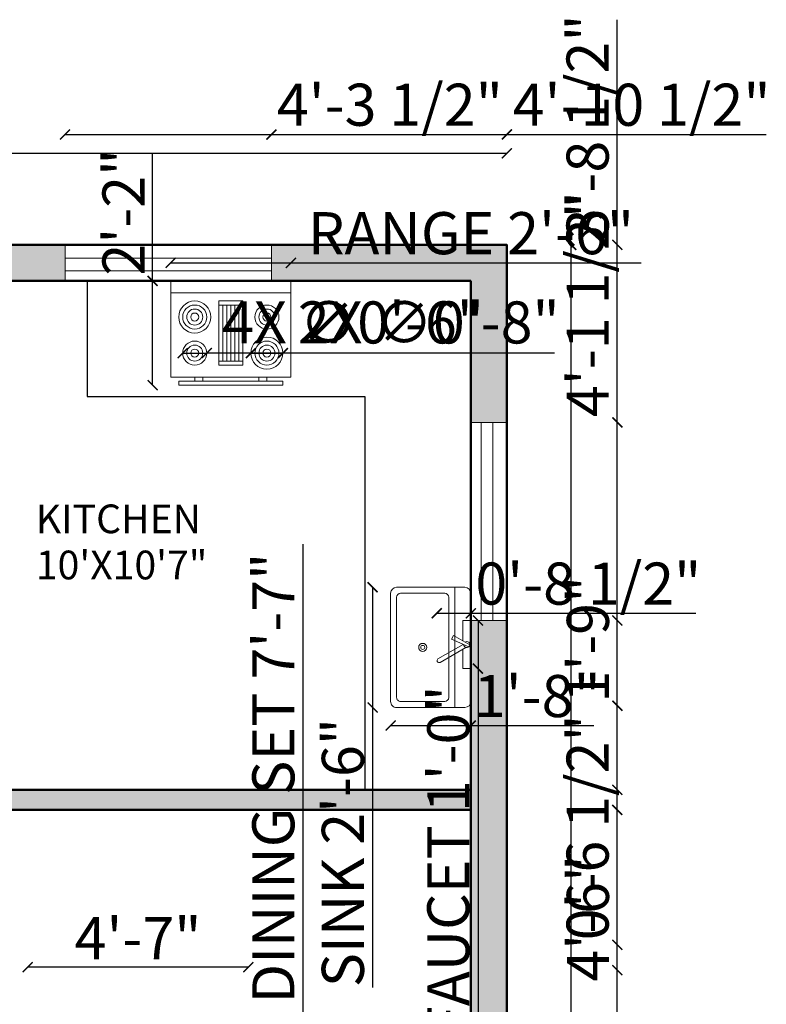
# Model space of a CAD drawing. Units: inches. Extents: x 1699 to 2290, y 1404 to 1978.
# Tile 4 of 4: x 2086 to 2273, y 1732 to 1978. Entities that reach past the tile are written whole.
import ezdxf

# ---------------------------------------------------------------- set-up
doc = ezdxf.new("R2010")
doc.units = ezdxf.units.IN
for name, color, linetype, lineweight in [('A-ANNO-DIMS', 2, 'Continuous', 18), ('A-AREA-IDEN', 7, 'Continuous', 25), ('A-EQPM', 8, 'Continuous', 18), ('A-FLOR-CASE', 8, 'Continuous', 25), ('A-FLOR-FIXT', 9, 'Continuous', 18), ('A-WALL', 7, 'Continuous', 50), ('A-WALL-PATT', 17, 'Continuous', 13), ('window', 3, 'Continuous', 18)]:
    doc.layers.add(name, color=color, linetype=linetype, lineweight=lineweight)
doc.styles.get("Standard").update_dxf_attribs({"font": 'arial.ttf'})
doc.dimstyles.new('ISO-25', dxfattribs={"dimtxt": 10.5, "dimasz": 2.5, "dimexe": 1.25, "dimexo": 0.625, "dimtad": 1, "dimdec": 0, "dimlunit": 4, "dimtxsty": 'Standard', "dimblk": 'ARCHTICK', "dimcen": 2.5, "dimse1": 1, "dimse2": 1, "dimclrd": 4, "dimclrt": 2, "dimadec": 0, "dimazin": 0, "dimtfac": 1, "dimtdec": 0, "dimtmove": 0, "dimatfit": 3, "dimfxl": 1, "dimarcsym": 0})

# ---------------------------------------------------------------- blocks, each defined once
blk = doc.blocks.new('Range-Oven - 30 in top')
for p, q in [((0, -3), (30, -3)), ((12, -6), (18, -6)), ((13, -20), (13, -6)), ((14, -6), (14, -20)), ((15, -20), (15, -6)), ((16, -6), (16, -20)), ((17, -20), (17, -6)), ((18, -20), (12, -20)), ((6, -24), (6, -25)), ((8, -25), (8, -24)), ((22, -25), (22, -24)), ((24, -24), (24, -25))]:
    blk.add_line(p, q)
for points in [[(0, -24), (0, 0), (30, 0), (30, -24)], [(12, -21), (12, -5), (18, -5), (18, -21)], [(2, -26), (2, -25), (28, -25), (28, -26)]]:
    blk.add_lwpolyline(points, close=True)
for centre, radius in [((6, -9), 4), ((6, -9), 3), ((6, -9), 2), ((24, -9), 3), ((24, -9), 2), ((6, -9), 1), ((24, -9), 1), ((24, -18), 4), ((6, -18), 3), ((6, -18), 2), ((6, -18), 1), ((24, -18), 3), ((24, -18), 2), ((24, -18), 1)]:
    blk.add_circle(centre, radius)
blk = doc.blocks.new('Sink-single - 30 in top')
blk.add_line((-15, -3.999996), (15, -3.999996))
for points in [[(-13.5, 0), (13.5, 0)], [(-15, -18.499996), (-15, -1.5)], [(15, -1.5), (15, -18.499996)], [(-13.5, -17.499996), (-13.5, -6.499996)], [(-12.5, -5.499996), (12.5, -5.499996)], [(13.5, -6.499996), (13.5, -17.499996)], [(12.5, -18.499996), (-12.5, -18.499996)], [(13.5, -19.999996), (-13.5, -19.999996)]]:
    blk.add_lwpolyline(points)
for radius in [1, 0.5]:
    blk.add_circle((0, -11.999996), radius)
for centre, radius, start, end in [((-13.5, -1.5), 1.5, 90, 180), ((13.5, -1.5), 1.5, 0, 90), ((-12.5, -6.499996), 1, 90, 180), ((12.5, -6.499996), 1, 0, 90), ((-13.5, -18.499996), 1.5, 180, 270), ((-12.5, -17.499996), 1, 180, 270), ((12.5, -17.499996), 1, 270, 0), ((13.5, -18.499996), 1.5, 270, 0)]:
    blk.add_arc(centre, radius, start, end)
blk = doc.blocks.new('Faucet - single handle top')
for p, q in [((0.08, -0.26), (-2.26, -4.34)), ((-1.37, -4.79), (0.55, -0.5)), ((-0.06, -1.9), (3.57, -8.18)), ((4.43, -7.68), (0.72, -1.24)), ((-2.26, -4.34), (-1.37, -4.79))]:
    blk.add_line(p, q)
for points in [[(-0.92, -2), (-6, -2), (-6, 0), (6, 0), (6, -2), (1.16, -2)], [(-0.01, -2), (-0.12, -2)]]:
    blk.add_lwpolyline(points)
for centre, radius, start, end in [((0, -1), 0.75, 269.2246, 216.2304), ((4, -7.93), 0.5, 210, 30)]:
    blk.add_arc(centre, radius, start, end)
blk = doc.blocks.new('_ArchTick')
at = {"color": 0, "linetype": 'ByBlock', "const_width": 0.15}
blk.add_lwpolyline([(-0.5, -0.5), (0.5, 0.5)], dxfattribs=at)
blk = doc.blocks.new('*D10')
at = {"layer": 'A-ANNO-DIMS', "color": 0, "lineweight": -2, "transparency": 16777216}
blk.add_line((1847.82, 1944.45), (2207.82, 1944.45), dxfattribs=at)
at = {"layer": 'Defpoints', "color": 0, "transparency": 16777216}
for p in [(2207.82, 1944.45), (1847.82, 1921.58), (2207.82, 1921.58)]:
    blk.add_point(p, dxfattribs=at)
at = {"layer": 'A-ANNO-DIMS', "color": 0, "lineweight": -2, "transparency": 16777216, "xscale": 2.5, "yscale": 2.5, "zscale": 2.5, "rotation": 180}
blk.add_blockref('_ArchTick', (1847.82, 1944.45), dxfattribs=at)
at = {"layer": 'A-ANNO-DIMS', "color": 0, "lineweight": -2, "transparency": 16777216, "xscale": 2.5, "yscale": 2.5, "zscale": 2.5}
blk.add_blockref('_ArchTick', (2207.82, 1944.45), dxfattribs=at)
at = {"layer": 'A-ANNO-DIMS', "color": 0, "transparency": 16777216, "insert": (2027.82, 1950.44), "char_height": 10.5, "attachment_point": 5}
blk.add_mtext("30'", dxfattribs=at)
blk = doc.blocks.new('*D11')
at = {"layer": 'A-ANNO-DIMS', "color": 0, "lineweight": -2, "transparency": 16777216}
blk.add_line((2223.88, 1441.58), (2223.88, 1921.58), dxfattribs=at)
at = {"layer": 'Defpoints', "color": 0, "transparency": 16777216}
for p in [(2207.82, 1921.58), (2223.88, 1921.58), (2207.82, 1441.58)]:
    blk.add_point(p, dxfattribs=at)
at = {"layer": 'A-ANNO-DIMS', "color": 0, "lineweight": -2, "transparency": 16777216, "xscale": 2.5, "yscale": 2.5, "zscale": 2.5}
for p, rotation in [((2223.88, 1921.58), 90), ((2223.88, 1441.58), 270)]:
    blk.add_blockref('_ArchTick', p, dxfattribs=dict(at, rotation=rotation))
at = {"layer": 'A-ANNO-DIMS', "color": 0, "transparency": 16777216, "insert": (2217.89, 1681.58), "char_height": 10.5, "attachment_point": 5, "rotation": 90}
blk.add_mtext("40'", dxfattribs=at)
blk = doc.blocks.new('*D16')
at = {"layer": 'A-ANNO-DIMS', "color": 4, "lineweight": -2, "transparency": 16777216}
for p, q in [((2156.97, 1727.7), (2156.97, 1846.86)), ((2156.97, 1636.7), (2156.97, 1727.7))]:
    blk.add_line(p, q, dxfattribs=at)
at = {"layer": 'Defpoints', "color": 0, "transparency": 16777216}
for p in [(2143.32, 1727.7), (2156.97, 1727.7), (2143.32, 1636.7)]:
    blk.add_point(p, dxfattribs=at)
at = {"layer": 'A-ANNO-DIMS', "color": 4, "lineweight": -2, "transparency": 16777216, "xscale": 2.5, "yscale": 2.5, "zscale": 2.5}
for p, rotation in [((2156.97, 1727.7), 90), ((2156.97, 1636.7), 270)]:
    blk.add_blockref('_ArchTick', p, dxfattribs=dict(at, rotation=rotation))
at = {"layer": 'A-ANNO-DIMS', "color": 2, "transparency": 16777216, "insert": (2150.92, 1788.53), "char_height": 10.5, "attachment_point": 5, "rotation": 90}
blk.add_mtext('DINING SET 7\'-7"', dxfattribs=at)
blk = doc.blocks.new('*D17')
at = {"layer": 'A-ANNO-DIMS', "color": 4, "lineweight": -2, "transparency": 16777216}
blk.add_line((2143.32, 1741.35), (2088.32, 1741.35), dxfattribs=at)
at = {"layer": 'Defpoints', "color": 0, "transparency": 16777216}
for p in [(2088.32, 1741.35), (2088.32, 1727.7), (2143.32, 1727.7)]:
    blk.add_point(p, dxfattribs=at)
at = {"layer": 'A-ANNO-DIMS', "color": 4, "lineweight": -2, "transparency": 16777216, "xscale": 2.5, "yscale": 2.5, "zscale": 2.5, "rotation": 180}
blk.add_blockref('_ArchTick', (2088.32, 1741.35), dxfattribs=at)
at = {"layer": 'A-ANNO-DIMS', "color": 4, "lineweight": -2, "transparency": 16777216, "xscale": 2.5, "yscale": 2.5, "zscale": 2.5}
blk.add_blockref('_ArchTick', (2143.32, 1741.35), dxfattribs=at)
at = {"layer": 'A-ANNO-DIMS', "color": 2, "transparency": 16777216, "insert": (2115.82, 1747.22), "char_height": 10.5, "attachment_point": 5}
blk.add_mtext('4\'-7"', dxfattribs=at)
blk = doc.blocks.new('*D18')
at = {"layer": 'A-ANNO-DIMS', "color": 4, "lineweight": -2, "transparency": 16777216}
for p, q in [((2123.96, 1917.08), (2153.96, 1917.08)), ((2153.96, 1917.08), (2241.31, 1917.08))]:
    blk.add_line(p, q, dxfattribs=at)
at = {"layer": 'Defpoints', "color": 0, "transparency": 16777216}
for p in [(2153.96, 1917.08), (2123.96, 1912.58), (2153.96, 1912.58)]:
    blk.add_point(p, dxfattribs=at)
at = {"layer": 'A-ANNO-DIMS', "color": 4, "lineweight": -2, "transparency": 16777216, "xscale": 2.5, "yscale": 2.5, "zscale": 2.5, "rotation": 180}
blk.add_blockref('_ArchTick', (2123.96, 1917.08), dxfattribs=at)
at = {"layer": 'A-ANNO-DIMS', "color": 4, "lineweight": -2, "transparency": 16777216, "xscale": 2.5, "yscale": 2.5, "zscale": 2.5}
blk.add_blockref('_ArchTick', (2153.96, 1917.08), dxfattribs=at)
at = {"layer": 'A-ANNO-DIMS', "color": 2, "transparency": 16777216, "insert": (2198.88, 1923.14), "char_height": 10.5, "attachment_point": 5}
blk.add_mtext('RANGE 2\'-6"', dxfattribs=at)
blk = doc.blocks.new('*D19')
at = {"layer": 'A-ANNO-DIMS', "color": 4, "lineweight": -2, "transparency": 16777216}
for p, q in [((2119.46, 1912.58), (2119.46, 1944.43)), ((2119.46, 1886.58), (2119.46, 1912.58))]:
    blk.add_line(p, q, dxfattribs=at)
at = {"layer": 'Defpoints', "color": 0, "transparency": 16777216}
for p in [(2119.46, 1912.58), (2123.96, 1912.58), (2123.96, 1886.58)]:
    blk.add_point(p, dxfattribs=at)
at = {"layer": 'A-ANNO-DIMS', "color": 4, "lineweight": -2, "transparency": 16777216, "xscale": 2.5, "yscale": 2.5, "zscale": 2.5}
for p, rotation in [((2119.46, 1912.58), 90), ((2119.46, 1886.58), 270)]:
    blk.add_blockref('_ArchTick', p, dxfattribs=dict(at, rotation=rotation))
at = {"layer": 'A-ANNO-DIMS', "color": 2, "transparency": 16777216, "insert": (2113.56, 1929.76), "char_height": 10.5, "attachment_point": 5, "rotation": 90}
blk.add_mtext('2\'-2"', dxfattribs=at)
blk = doc.blocks.new('*D20')
at = {"layer": 'A-ANNO-DIMS', "color": 4, "lineweight": -2, "transparency": 16777216}
for p, q in [((2174.32, 1836.15), (2174.32, 1806.15)), ((2174.32, 1806.15), (2174.32, 1736.23))]:
    blk.add_line(p, q, dxfattribs=at)
at = {"layer": 'Defpoints', "color": 0, "transparency": 16777216}
for p in [(2178.82, 1836.15), (2174.32, 1806.15), (2178.82, 1806.15)]:
    blk.add_point(p, dxfattribs=at)
at = {"layer": 'A-ANNO-DIMS', "color": 4, "lineweight": -2, "transparency": 16777216, "xscale": 2.5, "yscale": 2.5, "zscale": 2.5}
for p, rotation in [((2174.32, 1836.15), 90), ((2174.32, 1806.15), 270)]:
    blk.add_blockref('_ArchTick', p, dxfattribs=dict(at, rotation=rotation))
at = {"layer": 'A-ANNO-DIMS', "color": 2, "transparency": 16777216, "insert": (2168.27, 1769.94), "char_height": 10.5, "attachment_point": 5, "rotation": 90}
blk.add_mtext('SINK 2\'-6"', dxfattribs=at)
blk = doc.blocks.new('*D21')
at = {"layer": 'A-ANNO-DIMS', "color": 4, "lineweight": -2, "transparency": 16777216}
for p, q in [((2178.82, 1801.65), (2198.82, 1801.65)), ((2198.82, 1801.65), (2229.49, 1801.65))]:
    blk.add_line(p, q, dxfattribs=at)
at = {"layer": 'Defpoints', "color": 0, "transparency": 16777216}
for p in [(2178.82, 1806.15), (2198.82, 1806.15), (2198.82, 1801.65)]:
    blk.add_point(p, dxfattribs=at)
at = {"layer": 'A-ANNO-DIMS', "color": 4, "lineweight": -2, "transparency": 16777216, "xscale": 2.5, "yscale": 2.5, "zscale": 2.5, "rotation": 180}
blk.add_blockref('_ArchTick', (2178.82, 1801.65), dxfattribs=at)
at = {"layer": 'A-ANNO-DIMS', "color": 4, "lineweight": -2, "transparency": 16777216, "xscale": 2.5, "yscale": 2.5, "zscale": 2.5}
blk.add_blockref('_ArchTick', (2198.82, 1801.65), dxfattribs=at)
at = {"layer": 'A-ANNO-DIMS', "color": 2, "transparency": 16777216, "insert": (2215.41, 1807.64), "char_height": 10.5, "attachment_point": 5}
blk.add_mtext('1\'-8"', dxfattribs=at)
blk = doc.blocks.new('*D22')
at = {"layer": 'A-ANNO-DIMS', "color": 4, "lineweight": -2, "transparency": 16777216}
for p, q in [((2200.62, 1827.84), (2200.62, 1815.84)), ((2200.62, 1815.84), (2200.62, 1722.02))]:
    blk.add_line(p, q, dxfattribs=at)
at = {"layer": 'Defpoints', "color": 0, "transparency": 16777216}
for p in [(2198.82, 1827.84), (2198.82, 1815.84), (2200.62, 1815.84)]:
    blk.add_point(p, dxfattribs=at)
at = {"layer": 'A-ANNO-DIMS', "color": 4, "lineweight": -2, "transparency": 16777216, "xscale": 2.5, "yscale": 2.5, "zscale": 2.5}
for p, rotation in [((2200.62, 1827.84), 90), ((2200.62, 1815.84), 270)]:
    blk.add_blockref('_ArchTick', p, dxfattribs=dict(at, rotation=rotation))
at = {"layer": 'A-ANNO-DIMS', "color": 2, "transparency": 16777216, "insert": (2194.57, 1767.68), "char_height": 10.5, "attachment_point": 5, "rotation": 90}
blk.add_mtext('FAUCET 1\'-0"', dxfattribs=at)
blk = doc.blocks.new('*D23')
at = {"layer": 'A-ANNO-DIMS', "color": 4, "lineweight": -2, "transparency": 16777216}
for p, q in [((2190.32, 1829.64), (2198.82, 1829.64)), ((2198.82, 1829.64), (2254.95, 1829.64))]:
    blk.add_line(p, q, dxfattribs=at)
at = {"layer": 'Defpoints', "color": 0, "transparency": 16777216}
for p in [(2198.82, 1829.64), (2190.32, 1827.84), (2198.82, 1827.84)]:
    blk.add_point(p, dxfattribs=at)
at = {"layer": 'A-ANNO-DIMS', "color": 4, "lineweight": -2, "transparency": 16777216, "xscale": 2.5, "yscale": 2.5, "zscale": 2.5, "rotation": 180}
blk.add_blockref('_ArchTick', (2190.32, 1829.64), dxfattribs=at)
at = {"layer": 'A-ANNO-DIMS', "color": 4, "lineweight": -2, "transparency": 16777216, "xscale": 2.5, "yscale": 2.5, "zscale": 2.5}
blk.add_blockref('_ArchTick', (2198.82, 1829.64), dxfattribs=at)
at = {"layer": 'A-ANNO-DIMS', "color": 2, "transparency": 16777216, "insert": (2228.14, 1835.7), "char_height": 10.5, "attachment_point": 5}
blk.add_mtext('0\'-8 1/2"', dxfattribs=at)
blk = doc.blocks.new('*D40')
at = {"layer": 'A-ANNO-DIMS', "color": 4, "lineweight": -2, "transparency": 16777216}
blk.add_line((2235.37, 1726.54), (2235.37, 1780.58), dxfattribs=at)
at = {"layer": 'Defpoints', "color": 0, "transparency": 16777216}
for p in [(2198.82, 1780.58), (2235.37, 1780.58), (2207.82, 1726.54)]:
    blk.add_point(p, dxfattribs=at)
at = {"layer": 'A-ANNO-DIMS', "color": 4, "lineweight": -2, "transparency": 16777216, "xscale": 2.5, "yscale": 2.5, "zscale": 2.5}
for p, rotation in [((2235.37, 1780.58), 90), ((2235.37, 1726.54), 270)]:
    blk.add_blockref('_ArchTick', p, dxfattribs=dict(at, rotation=rotation))
at = {"layer": 'A-ANNO-DIMS', "color": 2, "transparency": 16777216, "insert": (2229.39, 1753.56), "char_height": 10.5, "attachment_point": 5, "rotation": 90}
blk.add_mtext('4\'-6"', dxfattribs=at)
blk = doc.blocks.new('*D42')
at = {"layer": 'A-ANNO-DIMS', "color": 4, "lineweight": -2, "transparency": 16777216}
for p, q in [((2172.42, 1414.03), (2198.82, 1414.03)), ((2198.82, 1414.03), (2255.13, 1414.03))]:
    blk.add_line(p, q, dxfattribs=at)
at = {"layer": 'Defpoints', "color": 0, "transparency": 16777216}
for p in [(2172.42, 1785.58), (2198.82, 1785.58), (2198.82, 1414.03)]:
    blk.add_point(p, dxfattribs=at)
at = {"layer": 'A-ANNO-DIMS', "color": 4, "lineweight": -2, "transparency": 16777216, "xscale": 2.5, "yscale": 2.5, "zscale": 2.5, "rotation": 180}
blk.add_blockref('_ArchTick', (2172.42, 1414.03), dxfattribs=at)
at = {"layer": 'A-ANNO-DIMS', "color": 4, "lineweight": -2, "transparency": 16777216, "xscale": 2.5, "yscale": 2.5, "zscale": 2.5}
blk.add_blockref('_ArchTick', (2198.82, 1414.03), dxfattribs=at)
at = {"layer": 'A-ANNO-DIMS', "color": 2, "transparency": 16777216, "insert": (2228.23, 1420.09), "char_height": 10.5, "attachment_point": 5}
blk.add_mtext('2\'-2 1/2"', dxfattribs=at)
blk = doc.blocks.new('*D43')
at = {"layer": 'A-ANNO-DIMS', "color": 4, "lineweight": -2, "transparency": 16777216}
for p, q in [((1768.27, 1912.58), (1768.27, 1883.78)), ((1768.27, 1883.78), (1768.27, 1851.94))]:
    blk.add_line(p, q, dxfattribs=at)
at = {"layer": 'Defpoints', "color": 0, "transparency": 16777216}
for p in [(2103.12, 1912.58), (1768.27, 1883.78), (2103.12, 1883.78)]:
    blk.add_point(p, dxfattribs=at)
at = {"layer": 'A-ANNO-DIMS', "color": 4, "lineweight": -2, "transparency": 16777216, "xscale": 2.5, "yscale": 2.5, "zscale": 2.5}
for p, rotation in [((1768.27, 1912.58), 90), ((1768.27, 1883.78), 270)]:
    blk.add_blockref('_ArchTick', p, dxfattribs=dict(at, rotation=rotation))
at = {"layer": 'A-ANNO-DIMS', "color": 2, "transparency": 16777216, "insert": (1762.29, 1866.61), "char_height": 10.5, "attachment_point": 5, "rotation": 90}
blk.add_mtext('2\'-5"', dxfattribs=at)
blk = doc.blocks.new('*D46')
at = {"layer": 'A-ANNO-DIMS', "color": 4, "lineweight": -2, "transparency": 16777216}
for p, q in [((2097.62, 1949.13), (2149.1, 1949.13)), ((2149.1, 1949.13), (2205.65, 1949.13))]:
    blk.add_line(p, q, dxfattribs=at)
at = {"layer": 'Defpoints', "color": 0, "transparency": 16777216}
for p in [(2149.1, 1949.13), (2097.62, 1921.58), (2149.1, 1921.58)]:
    blk.add_point(p, dxfattribs=at)
at = {"layer": 'A-ANNO-DIMS', "color": 4, "lineweight": -2, "transparency": 16777216, "xscale": 2.5, "yscale": 2.5, "zscale": 2.5, "rotation": 180}
blk.add_blockref('_ArchTick', (2097.62, 1949.13), dxfattribs=at)
at = {"layer": 'A-ANNO-DIMS', "color": 4, "lineweight": -2, "transparency": 16777216, "xscale": 2.5, "yscale": 2.5, "zscale": 2.5}
blk.add_blockref('_ArchTick', (2149.1, 1949.13), dxfattribs=at)
at = {"layer": 'A-ANNO-DIMS', "color": 2, "transparency": 16777216, "insert": (2178.63, 1955.19), "char_height": 10.5, "attachment_point": 5}
blk.add_mtext('4\'-3 1/2"', dxfattribs=at)
blk = doc.blocks.new('*D47')
at = {"layer": 'A-ANNO-DIMS', "color": 4, "lineweight": -2, "transparency": 16777216}
for p, q in [((2149.1, 1949.13), (2207.82, 1949.13)), ((2207.82, 1949.13), (2272.53, 1949.13))]:
    blk.add_line(p, q, dxfattribs=at)
at = {"layer": 'Defpoints', "color": 0, "transparency": 16777216}
for p in [(2207.82, 1949.13), (2149.1, 1921.58), (2207.82, 1921.58)]:
    blk.add_point(p, dxfattribs=at)
at = {"layer": 'A-ANNO-DIMS', "color": 4, "lineweight": -2, "transparency": 16777216, "xscale": 2.5, "yscale": 2.5, "zscale": 2.5, "rotation": 180}
blk.add_blockref('_ArchTick', (2149.1, 1949.13), dxfattribs=at)
at = {"layer": 'A-ANNO-DIMS', "color": 4, "lineweight": -2, "transparency": 16777216, "xscale": 2.5, "yscale": 2.5, "zscale": 2.5}
blk.add_blockref('_ArchTick', (2207.82, 1949.13), dxfattribs=at)
at = {"layer": 'A-ANNO-DIMS', "color": 2, "transparency": 16777216, "insert": (2241.43, 1955.19), "char_height": 10.5, "attachment_point": 5}
blk.add_mtext('4\'-10 1/2"', dxfattribs=at)
blk = doc.blocks.new('*D48')
at = {"layer": 'A-ANNO-DIMS', "color": 4, "lineweight": -2, "transparency": 16777216}
for p, q in [((2235.37, 1921.58), (2235.37, 1977.71)), ((2235.37, 1877.29), (2235.37, 1921.58))]:
    blk.add_line(p, q, dxfattribs=at)
at = {"layer": 'Defpoints', "color": 0, "transparency": 16777216}
for p in [(2207.82, 1921.58), (2235.37, 1921.58), (2207.82, 1877.29)]:
    blk.add_point(p, dxfattribs=at)
at = {"layer": 'A-ANNO-DIMS', "color": 4, "lineweight": -2, "transparency": 16777216, "xscale": 2.5, "yscale": 2.5, "zscale": 2.5}
for p, rotation in [((2235.37, 1921.58), 90), ((2235.37, 1877.29), 270)]:
    blk.add_blockref('_ArchTick', p, dxfattribs=dict(at, rotation=rotation))
at = {"layer": 'A-ANNO-DIMS', "color": 2, "transparency": 16777216, "insert": (2229.31, 1950.9), "char_height": 10.5, "attachment_point": 5, "rotation": 90}
blk.add_mtext('3\'-8 1/2"', dxfattribs=at)
blk = doc.blocks.new('*D49')
at = {"layer": 'A-ANNO-DIMS', "color": 4, "lineweight": -2, "transparency": 16777216}
for p, q in [((2235.37, 1877.29), (2235.37, 1933.84)), ((2235.37, 1827.84), (2235.37, 1877.29))]:
    blk.add_line(p, q, dxfattribs=at)
at = {"layer": 'Defpoints', "color": 0, "transparency": 16777216}
for p in [(2207.82, 1877.29), (2235.37, 1877.29), (2207.82, 1827.84)]:
    blk.add_point(p, dxfattribs=at)
at = {"layer": 'A-ANNO-DIMS', "color": 4, "lineweight": -2, "transparency": 16777216, "xscale": 2.5, "yscale": 2.5, "zscale": 2.5}
for p, rotation in [((2235.37, 1877.29), 90), ((2235.37, 1827.84), 270)]:
    blk.add_blockref('_ArchTick', p, dxfattribs=dict(at, rotation=rotation))
at = {"layer": 'A-ANNO-DIMS', "color": 2, "transparency": 16777216, "insert": (2229.32, 1906.82), "char_height": 10.5, "attachment_point": 5, "rotation": 90}
blk.add_mtext('4\'-1 1/2"', dxfattribs=at)
blk = doc.blocks.new('*D61')
at = {"layer": 'A-ANNO-DIMS', "color": 4, "lineweight": -2, "transparency": 16777216}
for p, q in [((2000.82, 1414.03), (2023.18, 1414.03)), ((2023.18, 1414.03), (2086.48, 1414.03))]:
    blk.add_line(p, q, dxfattribs=at)
at = {"layer": 'Defpoints', "color": 0, "transparency": 16777216}
for p in [(2000.82, 1842.58), (2023.18, 1842.58), (2023.18, 1414.03)]:
    blk.add_point(p, dxfattribs=at)
at = {"layer": 'A-ANNO-DIMS', "color": 4, "lineweight": -2, "transparency": 16777216, "xscale": 2.5, "yscale": 2.5, "zscale": 2.5, "rotation": 180}
blk.add_blockref('_ArchTick', (2000.82, 1414.03), dxfattribs=at)
at = {"layer": 'A-ANNO-DIMS', "color": 4, "lineweight": -2, "transparency": 16777216, "xscale": 2.5, "yscale": 2.5, "zscale": 2.5}
blk.add_blockref('_ArchTick', (2023.18, 1414.03), dxfattribs=at)
at = {"layer": 'A-ANNO-DIMS', "color": 2, "transparency": 16777216, "insert": (2056.08, 1420.09), "char_height": 10.5, "attachment_point": 5}
blk.add_mtext('1\'-10 1/2"', dxfattribs=at)
blk = doc.blocks.new('*D64')
at = {"layer": 'A-ANNO-DIMS', "color": 4, "lineweight": -2, "transparency": 16777216}
for p, q in [((2235.37, 1746.92), (2235.37, 1803.05)), ((2235.37, 1740.58), (2235.37, 1746.92))]:
    blk.add_line(p, q, dxfattribs=at)
at = {"layer": 'Defpoints', "color": 0, "transparency": 16777216}
for p in [(2005.82, 1746.92), (2235.37, 1746.92), (2000.82, 1740.58)]:
    blk.add_point(p, dxfattribs=at)
at = {"layer": 'A-ANNO-DIMS', "color": 4, "lineweight": -2, "transparency": 16777216, "xscale": 2.5, "yscale": 2.5, "zscale": 2.5}
for p, rotation in [((2235.37, 1746.92), 90), ((2235.37, 1740.58), 270)]:
    blk.add_blockref('_ArchTick', p, dxfattribs=dict(at, rotation=rotation))
at = {"layer": 'A-ANNO-DIMS', "color": 2, "transparency": 16777216, "insert": (2229.32, 1776.24), "char_height": 10.5, "attachment_point": 5, "rotation": 90}
blk.add_mtext('0\'-6 1/2"', dxfattribs=at)
blk = doc.blocks.new('*D67')
at = {"layer": 'A-ANNO-DIMS', "color": 4, "lineweight": -2, "transparency": 16777216}
for p, q in [((2075.82, 1414.03), (2103.12, 1414.03)), ((2103.12, 1414.03), (2159.43, 1414.03))]:
    blk.add_line(p, q, dxfattribs=at)
at = {"layer": 'Defpoints', "color": 0, "transparency": 16777216}
for p in [(2075.82, 1912.58), (2103.12, 1883.78), (2103.12, 1414.03)]:
    blk.add_point(p, dxfattribs=at)
at = {"layer": 'A-ANNO-DIMS', "color": 4, "lineweight": -2, "transparency": 16777216, "xscale": 2.5, "yscale": 2.5, "zscale": 2.5, "rotation": 180}
blk.add_blockref('_ArchTick', (2075.82, 1414.03), dxfattribs=at)
at = {"layer": 'A-ANNO-DIMS', "color": 4, "lineweight": -2, "transparency": 16777216, "xscale": 2.5, "yscale": 2.5, "zscale": 2.5}
blk.add_blockref('_ArchTick', (2103.12, 1414.03), dxfattribs=at)
at = {"layer": 'A-ANNO-DIMS', "color": 2, "transparency": 16777216, "insert": (2132.53, 1420.09), "char_height": 10.5, "attachment_point": 5}
blk.add_mtext('2\'-3 1/2"', dxfattribs=at)
blk = doc.blocks.new('*D68')
at = {"layer": 'A-ANNO-DIMS', "color": 4, "lineweight": -2, "transparency": 16777216}
for p, q in [((2103.12, 1414.03), (2123.96, 1414.03)), ((2123.96, 1414.03), (2154.63, 1414.03))]:
    blk.add_line(p, q, dxfattribs=at)
at = {"layer": 'Defpoints', "color": 0, "transparency": 16777216}
for p in [(2103.12, 1912.58), (2123.96, 1912.58), (2123.96, 1414.03)]:
    blk.add_point(p, dxfattribs=at)
at = {"layer": 'A-ANNO-DIMS', "color": 4, "lineweight": -2, "transparency": 16777216, "xscale": 2.5, "yscale": 2.5, "zscale": 2.5, "rotation": 180}
blk.add_blockref('_ArchTick', (2103.12, 1414.03), dxfattribs=at)
at = {"layer": 'A-ANNO-DIMS', "color": 4, "lineweight": -2, "transparency": 16777216, "xscale": 2.5, "yscale": 2.5, "zscale": 2.5}
blk.add_blockref('_ArchTick', (2123.96, 1414.03), dxfattribs=at)
at = {"layer": 'A-ANNO-DIMS', "color": 2, "transparency": 16777216, "insert": (2140.54, 1420.02), "char_height": 10.5, "attachment_point": 5}
blk.add_mtext('1\'-9"', dxfattribs=at)
blk = doc.blocks.new('*D69')
at = {"layer": 'A-ANNO-DIMS', "color": 4, "lineweight": -2, "transparency": 16777216}
for p, q in [((2235.37, 1806.59), (2235.37, 1837.26)), ((2235.37, 1785.58), (2235.37, 1806.59))]:
    blk.add_line(p, q, dxfattribs=at)
at = {"layer": 'Defpoints', "color": 0, "transparency": 16777216}
for p in [(2198.38, 1806.59), (2235.37, 1806.59), (2198.82, 1785.58)]:
    blk.add_point(p, dxfattribs=at)
at = {"layer": 'A-ANNO-DIMS', "color": 4, "lineweight": -2, "transparency": 16777216, "xscale": 2.5, "yscale": 2.5, "zscale": 2.5}
for p, rotation in [((2235.37, 1806.59), 90), ((2235.37, 1785.58), 270)]:
    blk.add_blockref('_ArchTick', p, dxfattribs=dict(at, rotation=rotation))
at = {"layer": 'A-ANNO-DIMS', "color": 2, "transparency": 16777216, "insert": (2229.39, 1823.18), "char_height": 10.5, "attachment_point": 5, "rotation": 90}
blk.add_mtext('1\'-9"', dxfattribs=at)
blk = doc.blocks.new('*D71')
at = {"layer": 'A-ANNO-DIMS', "color": 4, "lineweight": -2, "transparency": 16777216}
for p in [(2143.96, 1894.58), (2219.72, 1894.59)]:
    blk.add_line(p, (2151.96, 1894.59), dxfattribs=at)
at = {"layer": 'Defpoints', "color": 0, "transparency": 16777216}
for p in [(2143.96, 1894.58), (2151.96, 1894.59)]:
    blk.add_point(p, dxfattribs=at)
at = {"layer": 'A-ANNO-DIMS', "color": 4, "lineweight": -2, "transparency": 16777216, "xscale": 2.5, "yscale": 2.5, "zscale": 2.5}
for p, rotation in [((2143.96, 1894.58), 0.0016472536612344), ((2151.96, 1894.59), 180.0016472536612)]:
    blk.add_blockref('_ArchTick', p, dxfattribs=dict(at, rotation=rotation))
at = {"layer": 'A-ANNO-DIMS', "color": 2, "transparency": 16777216, "insert": (2188.34, 1900.87), "char_height": 10.5, "attachment_point": 5, "rotation": 0.0016}
blk.add_mtext('2X ∅0\'-8"', dxfattribs=at)
blk = doc.blocks.new('*D72')
at = {"layer": 'A-ANNO-DIMS', "color": 4, "lineweight": -2, "transparency": 16777216}
for p in [(2126.96, 1894.58), (2200.97, 1894.59)]:
    blk.add_line(p, (2132.96, 1894.59), dxfattribs=at)
at = {"layer": 'Defpoints', "color": 0, "transparency": 16777216}
for p in [(2126.96, 1894.58), (2132.96, 1894.59)]:
    blk.add_point(p, dxfattribs=at)
at = {"layer": 'A-ANNO-DIMS', "color": 4, "lineweight": -2, "transparency": 16777216, "xscale": 2.5, "yscale": 2.5, "zscale": 2.5}
for p, rotation in [((2126.96, 1894.58), 0.0021963382144996), ((2132.96, 1894.59), 180.0021963382145)]:
    blk.add_blockref('_ArchTick', p, dxfattribs=dict(at, rotation=rotation))
at = {"layer": 'A-ANNO-DIMS', "color": 2, "transparency": 16777216, "insert": (2169.46, 1900.87), "char_height": 10.5, "attachment_point": 5, "rotation": 0.0022}
blk.add_mtext('4X ∅0\'-6"', dxfattribs=at)

msp = doc.modelspace()

# ---------------------------------------------------------------- hatches: boundary and pattern name
at = {"layer": 'A-WALL-PATT'}
h = msp.add_hatch(color=256, dxfattribs=at)
h.dxf.hatch_style = 1
h.paths.add_polyline_path([(1893.7, 1921.58), (1847.82, 1921.58), (1847.82, 1852.66), (1856.82, 1852.66), (1856.82, 1912.58), (1893.7, 1912.58)])
h.paths.add_polyline_path([(2097.62, 1921.58), (1942.38, 1921.58), (1942.38, 1912.58), (2097.62, 1912.58)])
h.paths.add_polyline_path([(2207.82, 1921.58), (2149.1, 1921.58), (2149.1, 1912.58), (2153.96, 1912.58), (2198.82, 1912.58), (2198.82, 1877.29), (2207.82, 1877.29)])
h.paths.add_polyline_path([(2207.82, 1827.84), (2198.82, 1827.84), (2198.82, 1815.84), (2198.82, 1807.65), (2198.82, 1726.54), (2207.82, 1726.54)])
h.paths.add_polyline_path([(2207.82, 1677.38), (2198.82, 1677.38), (2198.82, 1660.38), (2198.82, 1547.09), (2207.82, 1547.09)])
h.paths.add_polyline_path([(2207.82, 1478.94), (2198.82, 1478.94), (2198.82, 1450.58), (1856.82, 1450.58), (1856.82, 1454.43), (1847.82, 1454.43), (1847.82, 1441.58), (2207.82, 1441.58)])
h.paths.add_polyline_path([(1856.82, 1567.67), (1847.82, 1567.67), (1847.82, 1476), (1856.82, 1476)])
h.paths.add_polyline_path([(1856.82, 1690.28), (1855.82, 1690.28), (1855.82, 1690.33), (1847.82, 1690.77), (1847.82, 1626.46), (1856.82, 1626.46)])
h.paths.add_polyline_path([(1856.82, 1802.75), (1847.82, 1802.75), (1847.82, 1720.13), (1856.82, 1720.13)])
h.paths.add_polyline_path([(2000.82, 1740.58), (1856.82, 1740.58), (1856.82, 1735.58), (2000.82, 1735.58)])
h.paths.add_polyline_path([(2005.82, 1668.58), (2000.82, 1668.58), (1856.82, 1668.58), (1856.82, 1663.58), (2000.82, 1663.58), (2000.82, 1644.06), (2005.82, 1644.06)])
h.paths.add_polyline_path([(2005.82, 1746.92), (2000.82, 1746.92), (2000.82, 1694.4), (2005.82, 1694.4)])
h.paths.add_polyline_path([(1957.82, 1735.58), (1952.82, 1735.58), (1952.82, 1694.4), (1957.82, 1694.4)])
h.paths.add_polyline_path([(2005.82, 1842.58), (2000.82, 1842.58), (2000.82, 1776.01), (2005.82, 1776.01)])
h.paths.add_polyline_path([(2000.82, 1519.58), (1911.72, 1519.58), (1911.72, 1514.58), (2000.82, 1514.58)])
h.paths.add_polyline_path([(1880.06, 1519.58), (1856.82, 1519.58), (1856.82, 1514.58), (1880.06, 1514.58)])
h.paths.add_polyline_path([(2005.82, 1615.11), (2000.82, 1615.11), (2000.82, 1519.58), (2005.82, 1519.58)])
h.paths.add_polyline_path([(2075.82, 1586.58), (2070.82, 1586.58), (2070.82, 1450.58), (2075.82, 1450.58)])
h.paths.add_polyline_path([(2198.82, 1591.58), (2112.54, 1591.58), (2112.54, 1586.58), (2198.82, 1586.58)])
h.paths.add_polyline_path([(2075.82, 1912.58), (2070.82, 1912.58), (2070.82, 1847.58), (2075.82, 1847.58)])
h.paths.add_polyline_path([(2198.82, 1785.58), (2075.82, 1785.58), (2075.82, 1780.58), (2198.82, 1780.58)])
h.paths.add_polyline_path([(2075.82, 1842.58), (2070.82, 1842.58), (2070.82, 1825.42), (2075.82, 1825.42)])
h.paths.add_polyline_path([(2075.82, 1847.58), (2070.82, 1847.58), (2070.82, 1842.58), (2075.82, 1842.58)])
h.paths.add_polyline_path([(2070.82, 1847.58), (2048.43, 1847.58), (2048.43, 1842.58), (2070.82, 1842.58)])
h.paths.add_polyline_path([(2023.18, 1847.58), (2005.82, 1847.58), (2005.82, 1842.58), (2023.18, 1842.58)])
h.paths.add_polyline_path([(2005.82, 1912.58), (2000.82, 1912.58), (2000.82, 1847.58), (2005.82, 1847.58)])
h.paths.add_polyline_path([(2005.82, 1847.58), (2000.82, 1847.58), (2000.82, 1842.58), (2005.82, 1842.58)])
h.paths.add_polyline_path([(2075.82, 1793.79), (2070.82, 1793.79), (2070.82, 1785.58), (2075.82, 1785.58)])
h.paths.add_polyline_path([(2075.82, 1785.58), (2070.82, 1785.58), (2070.82, 1780.58), (2075.82, 1780.58)])
h.paths.add_polyline_path([(2088.5, 1836.17), (2134.05, 1836.17), (2134.05, 1847.15), (2088.5, 1847.15)], flags=9)
h.paths.add_polyline_path([(2088.47, 1847.66), (2136.12, 1847.66), (2136.12, 1858.78), (2088.47, 1858.78)], flags=9)
h.paths.add_polyline_path([(2012.58, 1874.96), (2055.33, 1874.96), (2055.33, 1885.9), (2012.58, 1885.9)], flags=9)
h.paths.add_polyline_path([(2012.55, 1886.44), (2050.21, 1886.44), (2050.21, 1897.57), (2012.55, 1897.57)], flags=9)
h.paths.add_polyline_path([(1873.22, 1882.94), (1924.28, 1882.94), (1924.28, 1893.74), (1873.22, 1893.74)], flags=9)
h.paths.add_polyline_path([(1873.17, 1894.28), (1931.39, 1894.28), (1931.39, 1905.41), (1873.17, 1905.41)], flags=9)

# ---------------------------------------------------------------- linework, layer by layer
at = {"layer": 'A-FLOR-CASE'}
for p, q in [((2103.12, 1912.58), (2103.12, 1883.78)), ((2103.12, 1883.78), (2172.42, 1883.78)), ((2172.42, 1883.78), (2172.42, 1785.58))]:
    msp.add_line(p, q, dxfattribs=at)
at = {"layer": 'A-WALL'}
for p, q in [((1856.82, 1912.58), (2198.82, 1912.58)), ((2198.82, 1912.58), (2198.82, 1450.58)), ((2070.82, 1785.58), (2198.82, 1785.58)), ((2070.82, 1780.58), (2198.82, 1780.58))]:
    msp.add_line(p, q, dxfattribs=at)
msp.add_lwpolyline([(1847.82, 1921.58), (2207.82, 1921.58), (2207.82, 1441.58), (1847.82, 1441.58)], close=True, dxfattribs=at)
at = {"layer": 'window'}
for p, q in [((2097.62, 1921.58), (2097.62, 1912.58)), ((2149.1, 1921.58), (2097.62, 1921.58)), ((2149.1, 1912.58), (2149.1, 1921.58)), ((2149.1, 1918.26), (2097.62, 1918.26)), ((2149.1, 1915.12), (2097.62, 1915.12)), ((2097.62, 1912.58), (2149.1, 1912.58)), ((2207.82, 1877.29), (2198.82, 1877.29)), ((2198.82, 1877.29), (2198.82, 1827.84)), ((2201.41, 1877.29), (2201.41, 1827.84)), ((2204.32, 1877.29), (2204.32, 1827.84)), ((2207.82, 1827.84), (2207.82, 1877.29)), ((2198.82, 1827.84), (2207.82, 1827.84))]:
    msp.add_line(p, q, dxfattribs=at)

# ---------------------------------------------------------------- block references
at = {"layer": 'A-EQPM'}
msp.add_blockref('Range-Oven - 30 in top', (2123.96, 1912.58), dxfattribs=at)
at = {"layer": 'A-FLOR-FIXT', "rotation": 270}
for name, p in [('Sink-single - 30 in top', (2198.82, 1821.15)), ('Faucet - single handle top', (2198.82, 1821.84))]:
    msp.add_blockref(name, p, dxfattribs=at)

# ---------------------------------------------------------------- texts
at = {"layer": 'A-AREA-IDEN'}
for s, p in [('KITCHEN', (2090.32, 1849.63)), ('10\'X10\'7"', (2090.32, 1838.12))]:
    msp.add_text(s, height=7.167, dxfattribs=at).set_placement(p)

# ---------------------------------------------------------------- dimensions: what is measured, and where the dimension line sits
at = {"layer": 'A-ANNO-DIMS'}
for base, p1, p2, angle, override, picture, middle in [((2235.37, 1921.58), (2207.82, 1877.29), (2207.82, 1921.58), 90, {"dimdec": 1, "dimlfac": 1, "dimrnd": 0, "dimzin": 1, "dimdsep": 46, "dimlunit": 4, "dimfrac": 2}, '*D48', (2229.31, 1950.9)), ((2119.46, 1912.58), (2123.96, 1886.58), (2123.96, 1912.58), 90, {"dimdec": 1, "dimlfac": 1, "dimrnd": 0, "dimzin": 1, "dimdsep": 46, "dimlunit": 4, "dimfrac": 2}, '*D19', (2113.56, 1929.76)), ((2235.3716, 1877.2925), (2207.8216, 1827.8413), (2207.8216, 1877.2925), 90, {"dimdec": 1, "dimlfac": 1, "dimrnd": 0, "dimzin": 1, "dimdsep": 46, "dimlunit": 4, "dimfrac": 2}, '*D49', (2229.3176, 1906.8179)), ((2223.88, 1921.58), (2207.82, 1441.58), (2207.82, 1921.58), 90, {"dimclrd": 0, "dimclre": 0, "dimclrt": 0}, '*D11', (2217.89, 1681.58)), ((1768.27, 1883.78), (2103.12, 1912.58), (2103.12, 1883.78), 90, {"dimdec": 1, "dimlfac": 1, "dimrnd": 0, "dimzin": 1, "dimdsep": 46, "dimlunit": 4, "dimfrac": 2}, '*D43', (1762.29, 1866.61)), ((2235.37, 1806.59), (2198.82, 1785.58), (2198.38, 1806.59), 90, {"dimdec": 1, "dimlfac": 1, "dimrnd": 0, "dimzin": 1, "dimdsep": 46, "dimlunit": 4, "dimfrac": 2}, '*D69', (2229.39, 1823.18)), ((2235.37, 1746.92), (2000.82, 1740.58), (2005.82, 1746.92), 90, {"dimdec": 1, "dimlfac": 1, "dimrnd": 0, "dimzin": 1, "dimdsep": 46, "dimlunit": 4, "dimfrac": 2}, '*D64', (2229.32, 1776.24)), ((2235.37, 1780.58), (2207.82, 1726.54), (2198.82, 1780.58), 90, {"dimdec": 1, "dimlfac": 1, "dimrnd": 0, "dimzin": 1, "dimdsep": 46, "dimlunit": 4, "dimfrac": 2}, '*D40', (2229.39, 1753.56)), ((2088.32, 1741.35), (2143.32, 1727.7), (2088.32, 1727.7), 180, {"dimdec": 1, "dimlfac": 1, "dimrnd": 0, "dimzin": 1, "dimdsep": 46, "dimlunit": 4, "dimfrac": 2}, '*D17', (2115.82, 1747.22))]:
    dim = msp.add_linear_dim(base=base, p1=p1, p2=p2, angle=angle, dimstyle='ISO-25', override=override, dxfattribs=at)
    dim.commit()
    dim.dimension.update_dxf_attribs({"geometry": picture, "text_midpoint": middle})
for base, p1, p2, override, picture, middle in [((2149.1, 1949.13), (2097.62, 1921.58), (2149.1, 1921.58), {"dimdec": 1, "dimlfac": 1, "dimrnd": 0, "dimzin": 1, "dimdsep": 46, "dimlunit": 4, "dimfrac": 2}, '*D46', (2178.63, 1955.19)), ((2207.82, 1949.13), (2149.1, 1921.58), (2207.82, 1921.58), {"dimdec": 1, "dimlfac": 1, "dimrnd": 0, "dimzin": 1, "dimdsep": 46, "dimlunit": 4, "dimfrac": 2}, '*D47', (2241.43, 1955.19)), ((2207.82, 1944.45), (1847.82, 1921.58), (2207.82, 1921.58), {"dimclrd": 0, "dimclre": 0, "dimclrt": 0}, '*D10', (2027.82, 1950.44)), ((2103.12, 1414.03), (2075.82, 1912.58), (2103.12, 1883.78), {"dimdec": 1, "dimlfac": 1, "dimrnd": 0, "dimzin": 1, "dimdsep": 46, "dimlunit": 4, "dimfrac": 2}, '*D67', (2132.53, 1420.09)), ((2123.96, 1414.03), (2103.12, 1912.58), (2123.96, 1912.58), {"dimdec": 1, "dimlfac": 1, "dimrnd": 0, "dimzin": 1, "dimdsep": 46, "dimlunit": 4, "dimfrac": 2}, '*D68', (2140.54, 1420.02)), ((2198.82, 1829.64), (2190.32, 1827.84), (2198.82, 1827.84), {"dimdec": 1, "dimlfac": 1, "dimrnd": 0, "dimzin": 1, "dimdsep": 46, "dimlunit": 4, "dimfrac": 2}, '*D23', (2228.14, 1835.7)), ((2023.18, 1414.03), (2000.82, 1842.58), (2023.18, 1842.58), {"dimdec": 1, "dimlfac": 1, "dimrnd": 0, "dimzin": 1, "dimdsep": 46, "dimlunit": 4, "dimfrac": 2}, '*D61', (2056.08, 1420.09)), ((2198.82, 1801.65), (2178.82, 1806.15), (2198.82, 1806.15), {"dimdec": 1, "dimlfac": 1, "dimrnd": 0, "dimzin": 1, "dimdsep": 46, "dimlunit": 4, "dimfrac": 2}, '*D21', (2215.41, 1807.64)), ((2198.82, 1414.03), (2172.42, 1785.58), (2198.82, 1785.58), {"dimdec": 1, "dimlfac": 1, "dimrnd": 0, "dimzin": 1, "dimdsep": 46, "dimlunit": 4, "dimfrac": 2}, '*D42', (2228.23, 1420.09))]:
    dim = msp.add_linear_dim(base=base, p1=p1, p2=p2, dimstyle='ISO-25', override=override, dxfattribs=at)
    dim.commit()
    dim.dimension.update_dxf_attribs({"geometry": picture, "text_midpoint": middle})
dim = msp.add_linear_dim(base=(2153.96, 1917.08), p1=(2123.96, 1912.58), p2=(2153.96, 1912.58), text='RANGE <>', dimstyle='ISO-25', override={"dimdec": 1, "dimlfac": 1, "dimrnd": 0, "dimzin": 1, "dimdsep": 46, "dimlunit": 4, "dimfrac": 2}, dxfattribs=at)
dim.commit()
dim.dimension.update_dxf_attribs({"geometry": '*D18', "text_midpoint": (2198.88, 1923.14)})
dim = msp.add_diameter_dim_2p(p1=(2126.96, 1894.58), p2=(2132.96, 1894.59), text='4X <>', dimstyle='ISO-25', override={"dimdec": 1, "dimlfac": 1, "dimrnd": 0, "dimzin": 1, "dimdsep": 46, "dimlunit": 4, "dimfrac": 2}, dxfattribs=at)
dim.commit()
dim.dimension.update_dxf_attribs({"geometry": '*D72', "text_midpoint": (2169.46, 1894.59)})
dim = msp.add_diameter_dim_2p(p1=(2143.96, 1894.58), p2=(2151.96, 1894.59), text='2X <>', dimstyle='ISO-25', override={"dimdec": 1, "dimlfac": 1, "dimrnd": 0, "dimzin": 1, "dimdsep": 46, "dimlunit": 4, "dimfrac": 2}, dxfattribs=at)
dim.commit()
dim.dimension.update_dxf_attribs({"geometry": '*D71', "text_midpoint": (2188.34, 1894.59), "dimtype": 163})
for base, p1, p2, angle, text, picture, middle in [((2156.97, 1727.7), (2143.32, 1636.7), (2143.32, 1727.7), 90, 'DINING SET <>', '*D16', (2150.92, 1788.53)), ((2174.32, 1806.15), (2178.82, 1836.15), (2178.82, 1806.15), 270, 'SINK <>', '*D20', (2168.27, 1769.94)), ((2200.62, 1815.84), (2198.82, 1827.84), (2198.82, 1815.84), 270, 'FAUCET <>', '*D22', (2194.57, 1767.68))]:
    dim = msp.add_linear_dim(base=base, p1=p1, p2=p2, angle=angle, text=text, dimstyle='ISO-25', override={"dimdec": 1, "dimlfac": 1, "dimrnd": 0, "dimzin": 1, "dimdsep": 46, "dimlunit": 4, "dimfrac": 2}, dxfattribs=at)
    dim.commit()
    dim.dimension.update_dxf_attribs({"geometry": picture, "text_midpoint": middle})

doc.saveas('drawing.dxf')
